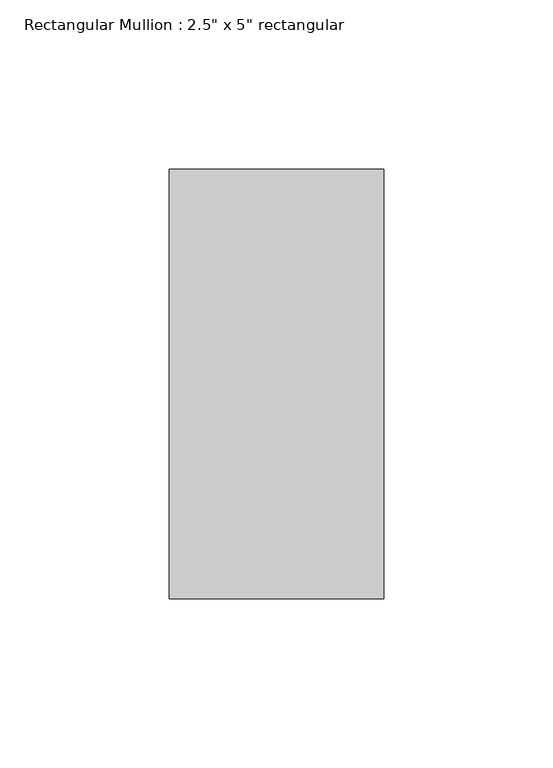
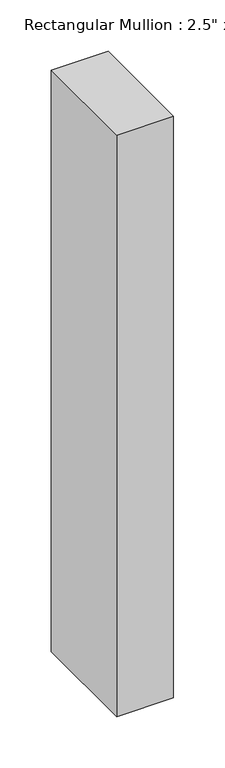
"""IFC4 building model written with IfcOpenShell, lengths in millimetres: member geometry."""

from ifc_helpers import new_model, si_unit, frame, origin, place, context, project, spatial, polyline, outline, extrude, source, transform, mapped, element, save


def member_3af75de8(model_context):
    return source(origin(), model_context, "Body", "SweptSolid", [
        extrude(outline(polyline([(31.75, 63.5), (31.75, -63.5), (-31.75, -63.5), (-31.75, 63.5), (31.75, 63.5)])), frame((0.0, 0.0, -689.6941631), z_axis=(0.0, 0.0, 1.0), x_axis=(1.0, 0.0, 0.0)), (0.0, 0.0, 1.0), 689.6941631),
    ])


if __name__ == "__main__":
    model = new_model("IFC4")
    model_context = context("Model", 3, world=origin())
    ifc_project = project(units=[si_unit("LENGTHUNIT", "METRE", prefix="MILLI")], contexts=[model_context])
    site = spatial("IfcSite", under=ifc_project)
    building = spatial("IfcBuilding", under=site)
    placement = place(None, origin())
    member_shape = member_3af75de8(model_context)
    element("IfcMember", 1, ObjectType="Rectangular Mullion : 2.5\" x 5\" rectangular", at=placement, inside=building, context=model_context, shape_type="MappedRepresentation", body=[
        mapped(member_shape, transform((0.0, 0.0, 0.0), x_axis=(1.0, 0.0, 0.0), y_axis=(0.0, 1.0, 0.0), z_axis=(0.0, 0.0, 1.0))),
    ])
    save(model, "model.ifc")

# Revit data of these elements
# Type "Rectangular Mullion : 2.5\" x 5\" rectangular"
#   built-in parameter 1007304 = 0.416667 (stored number, unit not read)
#   built-in parameter 1007301 = 0.104167 (stored number, unit not read)
#   built-in parameter 1007300 = 0.104167 (stored number, unit not read)
# Element 1 (IfcMember, "Rectangular Mullion : 2.5\" x 5\" rectangular")
#   Materials on its faces: "Aluminum"
# Materials
#   "Aluminum": class "Metal", colour RGB 247 247 247, transparency 0, Description = "Aluminum 6061", Cost = 0
